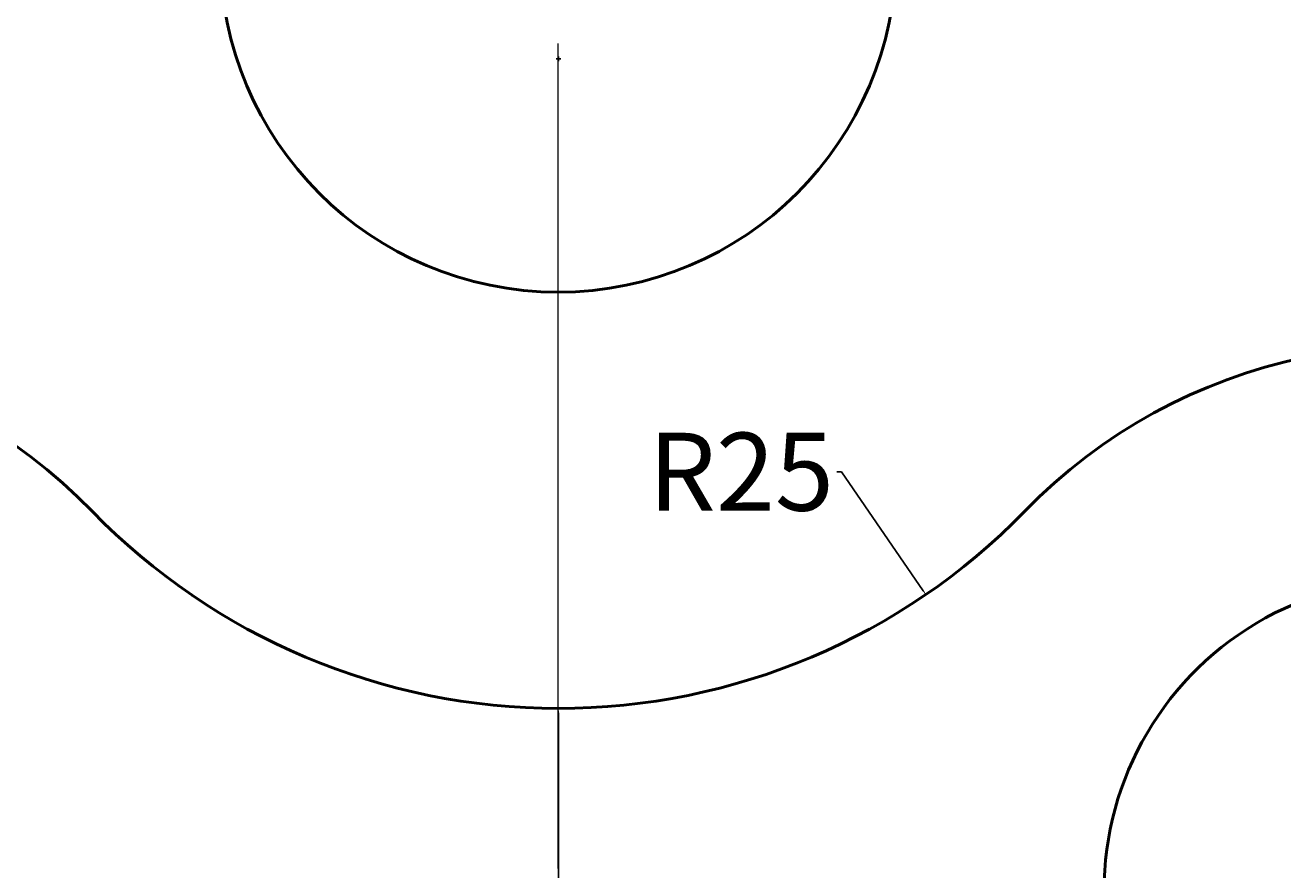
# Model space of a CAD drawing. Units: millimetres. Extents: x -50 to 109, y -46 to 152.
# Tile 13 of 18: x 13 to 61, y 67 to 100. Entities that reach past the tile are written whole.
import ezdxf

# ---------------------------------------------------------------- set-up
doc = ezdxf.new("R2010")
doc.units = ezdxf.units.MM
doc.header["$MEASUREMENT"] = 0
doc.linetypes.add('CENTER', pattern=[50.8, 31.75, -6.35, 6.35, -6.35])
for name, color, linetype, lineweight in [('M-CNTR', 1, 'CENTER', 18), ('M-DIMS', 2, 'Continuous', 25), ('M-OUTL', 7, 'Continuous', 50)]:
    doc.layers.add(name, color=color, linetype=linetype, lineweight=lineweight)
doc.styles.get("Standard").update_dxf_attribs({"font": 'arial.ttf'})
doc.dimstyles.get("Standard").update_dxf_attribs({"dimtxt": 0.18, "dimasz": 0.18, "dimexe": 0.18, "dimexo": 0.0625, "dimgap": 0.09, "dimtad": 0, "dimtih": 1, "dimtoh": 1, "dimdec": 4, "dimzin": 0, "dimdsep": 46, "dimtxsty": 'Standard', "dimcen": 0.09, "dimadec": 0, "dimazin": 0, "dimtfac": 1, "dimtdec": 4, "dimtofl": 0, "dimtmove": 0, "dimatfit": 3, "dimfxl": 1, "dimtolj": 1, "dimtzin": 0, "dimarcsym": 0})

# ---------------------------------------------------------------- blocks, each defined once
blk = doc.blocks.new('*U3')
at = {"layer": 'M-CNTR', "color": 0, "transparency": 16777216}
blk.add_line((0, -85.984), (0, -2.6), dxfattribs=at)
blk = doc.blocks.new('*D11')
at = {"layer": 'Defpoints', "color": 0, "transparency": 16777216}
for p in [(29.306, 114.679), (36.932, 89.822)]:
    blk.add_point(p, dxfattribs=at)
at = {"layer": 'M-DIMS', "color": 0, "lineweight": -2, "transparency": 16777216}
for p, q in [((25.349, 126.988), (25.529, 126.988)), ((25.529, 126.988), (29.253, 114.851)), ((33.029, 102.251), (33.209, 102.251)), ((33.119, 102.161), (33.119, 102.341))]:
    blk.add_line(p, q, dxfattribs=at)
at = {"layer": 'M-DIMS', "color": 0, "transparency": 16777216}
blk.add_solid([(29.282, 114.86), (29.224, 114.842), (29.306, 114.679)], dxfattribs=at)
at = {"layer": 'M-DIMS', "color": 0, "transparency": 16777216, "insert": (21.48, 126.988), "char_height": 0.18, "attachment_point": 5}
blk.add_mtext('\\A1;{\\H16.66667x;%%C26}', dxfattribs=at)
blk = doc.blocks.new('*D16')
at = {"layer": 'Defpoints', "color": 0, "transparency": 16777216}
for p in [(33.132, 98.231), (47.269, 77.612)]:
    blk.add_point(p, dxfattribs=at)
at = {"layer": 'M-DIMS', "color": 0, "lineweight": -2, "transparency": 16777216}
for p, q in [((43.847, 82.341), (44.027, 82.341)), ((44.027, 82.341), (47.167, 77.76))]:
    blk.add_line(p, q, dxfattribs=at)
at = {"layer": 'M-DIMS', "color": 0, "transparency": 16777216}
blk.add_solid([(47.192, 77.777), (47.142, 77.743), (47.269, 77.612)], dxfattribs=at)
at = {"layer": 'M-DIMS', "color": 0, "transparency": 16777216, "insert": (40.161, 82.341), "char_height": 0.18, "attachment_point": 5}
blk.add_mtext('\\A1;{\\H16.66667x;R25}', dxfattribs=at)
blk = doc.blocks.new('*D37')
at = {"layer": 'Defpoints', "color": 0, "transparency": 16777216}
for p in [(33.132, 98.231), (33.131, 73.231)]:
    blk.add_point(p, dxfattribs=at)
at = {"layer": 'M-DIMS', "color": 0, "lineweight": -2, "transparency": 16777216}
for p, q in [((33.132, 98.141), (33.132, 98.321)), ((33.042, 98.231), (33.222, 98.231)), ((33.13, 58.231), (33.131, 73.051)), ((32.95, 58.231), (33.13, 58.231))]:
    blk.add_line(p, q, dxfattribs=at)
at = {"layer": 'M-DIMS', "color": 0, "transparency": 16777216}
blk.add_solid([(33.101, 73.051), (33.161, 73.051), (33.131, 73.231)], dxfattribs=at)
at = {"layer": 'M-DIMS', "color": 0, "transparency": 16777216, "insert": (32.645, 58.231), "char_height": 0.18, "attachment_point": 5}
blk.add_mtext('\\A1;R25', dxfattribs=at)

msp = doc.modelspace()

# ---------------------------------------------------------------- linework, layer by layer
at = {"layer": 'M-OUTL'}
msp.add_circle((33.11888, 102.25066), 13, dxfattribs=at)
for centre, radius, start, end in [((0.13105, 66.18507), 21, 44.15899, 179.845381), ((66.1299, 66.18218), 21, 0.162515, 135.835986), ((33.13188, 98.23105), 25, 224.15899, 315.835986), ((66.12325, 66.19749), 12, 0.211276, 183.937929)]:
    msp.add_arc(centre, radius, start, end, dxfattribs=at)

# ---------------------------------------------------------------- block references
at = {"layer": 'M-CNTR'}
msp.add_blockref('*U3', (33.11888, 102.25066), dxfattribs=at)

# ---------------------------------------------------------------- dimensions: what is measured, and where the dimension line sits
at = {"layer": 'M-DIMS'}
dim = msp.add_diameter_dim_2p(p1=(36.93188, 89.82243), p2=(29.30587, 114.6789), text='{\\H16.66667x;%%C26}', dimstyle='Standard', override={"dimclrd": 0, "dimclre": 0, "dimclrt": 0}, dxfattribs=at)
dim.commit()
dim.dimension.update_dxf_attribs({"geometry": '*D11', "text_midpoint": (21.47969, 126.98819), "dimtype": 163})
dim = msp.add_radius_dim(center=(33.13188, 98.23105), mpoint=(33.131, 73.23105), dimstyle='Standard', override={"dimdec": 0, "dimlfac": 1, "dimrnd": 0, "dimzin": 0, "dimdsep": 46, "dimlunit": 2}, dxfattribs=at)
dim.commit()
dim.dimension.update_dxf_attribs({"geometry": '*D37', "text_midpoint": (32.64474, 58.23105), "dimtype": 164})
dim = msp.add_radius_dim(center=(33.13188, 98.23105), mpoint=(47.2688, 77.61195), text='{\\H16.66667x;R25}', dimstyle='Standard', override={"dimclrd": 0, "dimclre": 0, "dimclrt": 0}, dxfattribs=at)
dim.commit()
dim.dimension.update_dxf_attribs({"geometry": '*D16', "text_midpoint": (40.16119, 82.34067), "dimtype": 164})

doc.saveas('drawing.dxf')
